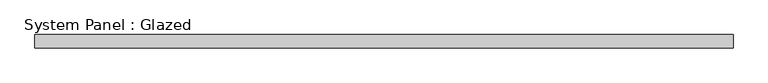
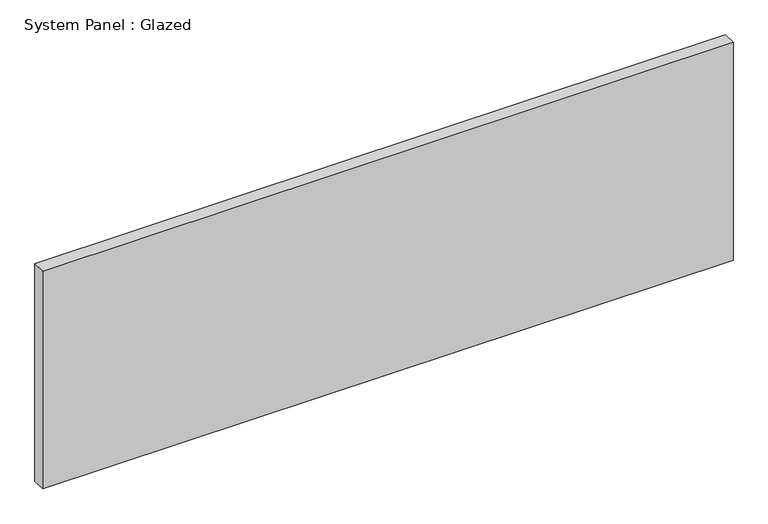
"""IFC4 building model written with IfcOpenShell, lengths in millimetres: plate geometry, System Panel : Glazed."""

from ifc_helpers import new_model, si_unit, origin, origin_with_axes, place, context, project, spatial, polyline, outline, extrude, source, transform, mapped, element, save


def system_panel_glazed_1cb66d18(model_context):
    return source(origin(), model_context, "Body", "SweptSolid", [
        extrude(outline(polyline([(666.7499999, -44.45), (-666.7499999, -44.45), (-666.7499999, -19.05), (666.7499999, -19.05), (666.7499999, -44.45)])), origin_with_axes(), (0.0, 0.0, 1.0), 444.5),
    ])


if __name__ == "__main__":
    model = new_model("IFC4")
    model_context = context("Model", 3, world=origin())
    ifc_project = project(units=[si_unit("LENGTHUNIT", "METRE", prefix="MILLI")], contexts=[model_context])
    site = spatial("IfcSite", under=ifc_project)
    building = spatial("IfcBuilding", under=site)
    placement = place(None, origin())
    system_panel_glazed_shape = system_panel_glazed_1cb66d18(model_context)
    element("IfcPlate", 1, ObjectType="System Panel : Glazed", at=placement, inside=building, context=model_context, shape_type="MappedRepresentation", body=[
        mapped(system_panel_glazed_shape, transform((0.0, 0.0, 0.0), x_axis=(1.0, 0.0, 0.0), y_axis=(0.0, 1.0, 0.0), z_axis=(0.0, 0.0, 1.0))),
    ])
    save(model, "model.ifc")

# Revit data of these elements
# Type "System Panel : Glazed"
#   Construction Type Id = "GSP4R"
#   Analytic Construction = "1/8 in Pilkington single glazing"
#   Visual Light Transmittance = 0.9
#   Solar Heat Gain Coefficient = 0.86
#   Heat Transfer Coefficient (U) = 1.18115 BTU/(h·ft²·°F)
#   Define Thermal Properties by = 1
# Element 1 (IfcPlate, "System Panel : Glazed")
#   Materials on its faces: "glass panel 223"
# Materials
#   "glass panel 223": class "Generic", colour RGB 120 120 120, transparency 0, Cost = 0
